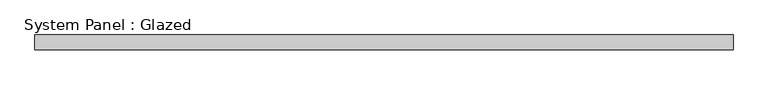
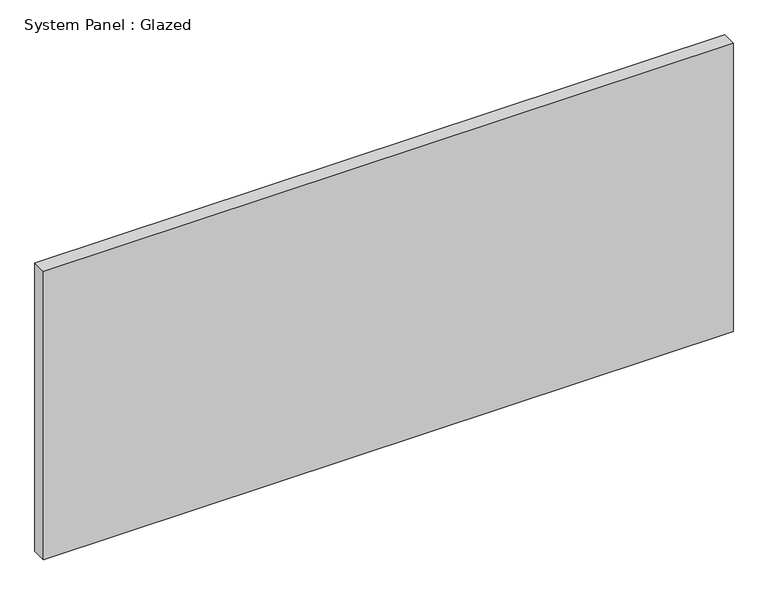
"""IFC4 building model written with IfcOpenShell, lengths in millimetres: plate geometry, System Panel : Glazed."""

from ifc_helpers import new_model, si_unit, origin, origin_with_axes, place, context, project, spatial, polyline, outline, extrude, source, transform, mapped, element, save


def system_panel_glazed_3aabc813(model_context):
    return source(origin(), model_context, "Body", "SweptSolid", [
        extrude(outline(polyline([(597.5350001, 19.05), (-597.5350001, 19.05), (-597.5350001, 44.45), (597.5350001, 44.45), (597.5350001, 19.05)])), origin_with_axes(), (0.0, 0.0, 1.0), 528.4534682),
    ])


if __name__ == "__main__":
    model = new_model("IFC4")
    model_context = context("Model", 3, world=origin())
    ifc_project = project(units=[si_unit("LENGTHUNIT", "METRE", prefix="MILLI")], contexts=[model_context])
    site = spatial("IfcSite", under=ifc_project)
    building = spatial("IfcBuilding", under=site)
    placement = place(None, origin())
    system_panel_glazed_shape = system_panel_glazed_3aabc813(model_context)
    element("IfcPlate", 1, ObjectType="System Panel : Glazed", at=placement, inside=building, context=model_context, shape_type="MappedRepresentation", body=[
        mapped(system_panel_glazed_shape, transform((0.0, 0.0, 0.0), x_axis=(1.0, 0.0, 0.0), y_axis=(0.0, 1.0, 0.0), z_axis=(0.0, 0.0, 1.0))),
    ])
    save(model, "model.ifc")

# Revit data of these elements
# Type "System Panel : Glazed"
#   Construction Type Id = "GSP4R"
#   Analytic Construction = "1/8 in Pilkington single glazing"
#   Visual Light Transmittance = 0.9
#   Solar Heat Gain Coefficient = 0.86
#   Heat Transfer Coefficient (U) = 1.18115 BTU/(h·ft²·°F)
#   Define Thermal Properties by = 1
# Element 1 (IfcPlate, "System Panel : Glazed")
#   Materials on its faces: "Glass"
# Materials
#   "Glass": class "Glass", colour RGB 0 128 192, transparency 0.75, Description = "Soda Lime Glass", Cost = 0
